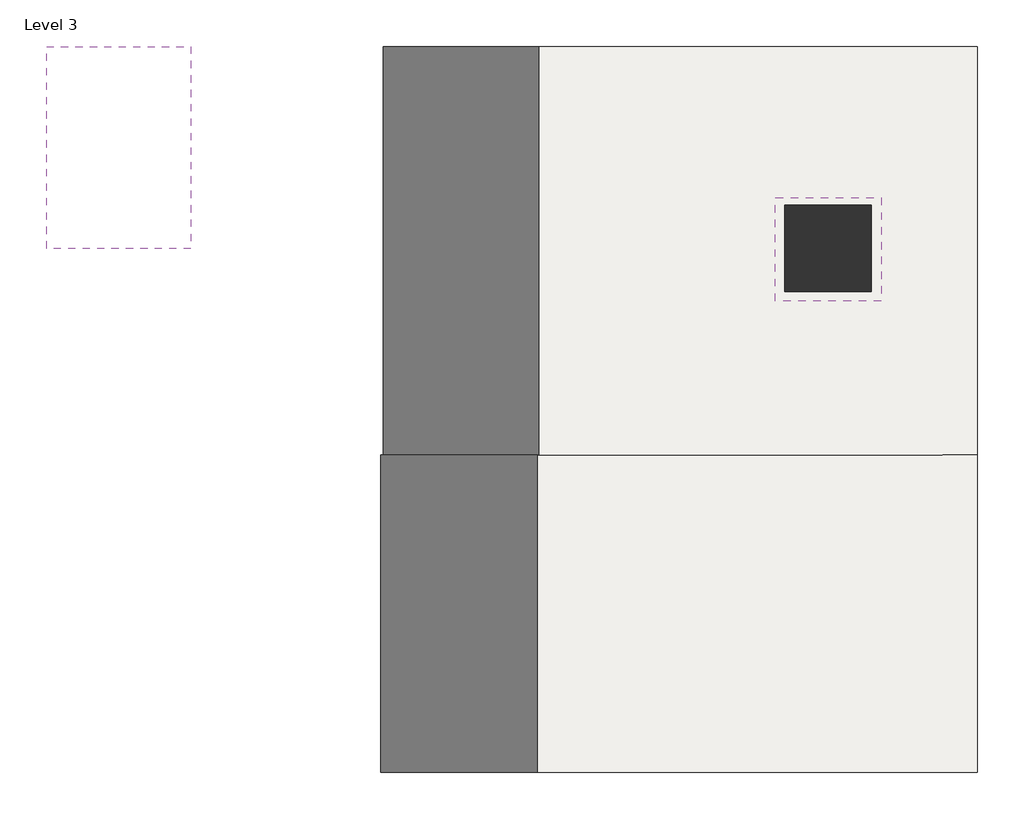
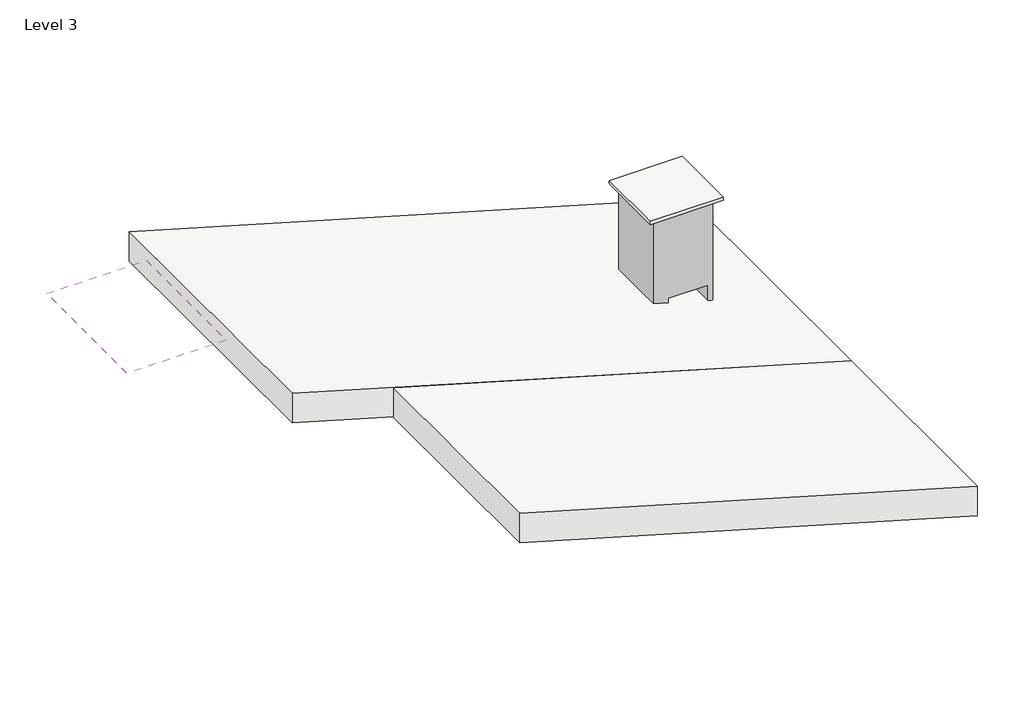
# One storey: 3 roofs, 1 column, 1 slab.
"""IFC4 building model written with IfcOpenShell, lengths in millimetres."""

from ifc_helpers import new_model, si_unit, frame, origin, place, context, project, spatial, polyline, outline, extrude, element, save

model = new_model("IFC4")

# Units and contexts
model_context = context("Model", 3, world=origin())
ifc_project = project(units=[si_unit("LENGTHUNIT", "METRE", prefix="MILLI")], contexts=[model_context])

# Site, building, storey
site = spatial("IfcSite", under=ifc_project)
building = spatial("IfcBuilding", under=site)
storey = spatial("IfcBuildingStorey", under=building, Name="Level 3", Elevation=5181.6)

# Column
placement = place(None, origin())
element("IfcColumn", 1, ObjectType="Rectangular Column : 24\" x 24\" 2", at=placement, inside=storey, context=model_context, shape_type="SweptSolid", body=[
    extrude(outline(polyline([(7010.4, -14282.2613196), (5181.6, -14282.2613196), (5181.6, -14053.6613196), (5638.8, -14053.6613196), (5638.8, -13444.0613196), (5181.6, -13444.0613196), (5181.6, -13367.8613196), (7010.4, -13367.8613196), (7010.4, -14282.2613196)])), frame((0.0, -279.8582127, 0.0), z_axis=(0.0, 1.0, 0.0), x_axis=(0.0, 0.0, 1.0)), (0.0, 0.0, 1.0), 914.4),
])

# Roofs
element("IfcRoof", 2, ObjectType="Generic - 18\"", at=placement, inside=storey, context=model_context, shape_type="SweptSolid", body=[
    extrude(outline(polyline([(5047.6877785, -12248.68247), (7061.3825559, -19259.08247), (6585.6947773, -19259.08247), (4572.0, -12248.68247), (5047.6877785, -12248.68247)])), frame((0.0, -5359.8582127, 0.0), z_axis=(0.0, 1.0, 0.0), x_axis=(0.0, 0.0, 1.0)), (0.0, 0.0, 1.0), 3352.8),
])
element("IfcRoof", 3, ObjectType="Generic - 18\"", at=placement, inside=storey, context=model_context, shape_type="SweptSolid", body=[
    extrude(outline(polyline([(5047.8158981, -12248.68247), (7515.766207, -20810.3057456), (7039.9503089, -20810.3057456), (4572.0, -12248.68247), (5047.8158981, -12248.68247)])), frame((0.0, -2007.0582127, 0.0), z_axis=(0.0, 1.0, 0.0), x_axis=(0.0, 0.0, 1.0)), (0.0, 0.0, 1.0), 4318.0),
])
element("IfcRoof", 4, ObjectType="Generic - 18\"", at=placement, inside=storey, context=model_context, shape_type="SweptSolid", body=[
    extrude(outline(polyline([(7441.3615965, -20556.0613196), (7947.571872, -22080.0613196), (7465.8102755, -22080.0613196), (6959.6, -20556.0613196), (7441.3615965, -20556.0613196)])), frame((0.0, 177.3417873, 0.0), z_axis=(0.0, 1.0, 0.0), x_axis=(0.0, 0.0, 1.0)), (0.0, 0.0, 1.0), 2133.6),
])

# Slab
element("IfcSlab", 5, ObjectType="Generic - 12\" 2", at=placement, inside=storey, context=model_context, shape_type="SweptSolid", body=[
    extrude(outline(polyline([(-13264.463748, 713.3946973), (-13264.463748, -378.8053027), (-14382.063748, -378.8053027), (-14382.063748, 713.3946973), (-13264.463748, 713.3946973)])), frame((0.0, 0.0, 7010.4), z_axis=(0.0, 0.0, 1.0), x_axis=(1.0, 0.0, 0.0)), (0.0, 0.0, 1.0), 50.8),
])

save(model, "model.ifc")

# Revit data of these elements
# Type "Rectangular Column : 24\" x 24\" 2"
#   Assembly Code = "B1010200"
#   Depth = 3' - 0"
#   Offset Base = 0' - 0"
#   Offset Top = 0' - 0"
#   Width = 3' - 0"
#   Material = Iron, Ductile
# Type "Generic - 18\""
#   Assembly Code = "B1020"
#   Layers, outside or top first: 1' - 6" "Stainless Steel" (function 1)
# Type "Generic - 12\" 2"
#   Assembly Code = "B1010"
#   Function = 0
#   Layers, outside or top first: 0' - 2" "Vinyl Composition Tile" (function 1)
# Element 1 (IfcColumn, "Rectangular Column : 24\" x 24\" 2")
#   Phase Created = New Construction
#   Materials on its faces: "Iron, Ductile", "Rigid insulation", "Brick, Soldier Course", "Oak Flooring"
# Element 2 (IfcRoof, "Generic - 18\"")
#   built-in parameter 1001705 = 23.1673 (stored number, unit not read)
#   built-in parameter 1001701 = -2 (stored number, unit not read)
#   built-in parameter 1001710 = 33615
#   Phase Created = New Construction
#   Materials on its faces: "Stainless Steel"
# Element 3 (IfcRoof, "Generic - 18\"")
#   built-in parameter 1001705 = 24.658 (stored number, unit not read)
#   built-in parameter 1001701 = -2 (stored number, unit not read)
#   built-in parameter 1001710 = 33615
#   Phase Created = New Construction
#   Materials on its faces: "Stainless Steel"
# Element 4 (IfcRoof, "Generic - 18\"")
#   built-in parameter 1001705 = 26.0747 (stored number, unit not read)
#   built-in parameter 1001701 = 5.83333 (stored number, unit not read)
#   built-in parameter 1001710 = 33615
#   Phase Created = New Construction
#   Materials on its faces: "Stainless Steel"
# Element 5 (IfcSlab, "Generic - 12\" 2")
#   Height Offset From Level = 6' - 2"
#   Phase Created = New Construction
#   Materials on its faces: "Vinyl Composition Tile"
# Materials
#   "Iron, Ductile": class "Metal", colour RGB 0 0 0, transparency 0, Description = "Ductile cast iron", Cost = 0
#   "Stainless Steel": class "Metal", colour RGB 0 0 0, transparency 0, Description = "Stainless Steel 18/8", Cost = 0
#   "Vinyl Composition Tile": class "Generic", colour RGB 179 160 124, transparency 0, Description = "Vinyl Composition Tile", Cost = 0
#   "Rigid insulation": class "Generic", colour RGB 127 127 127, transparency 0, Description = "Rigid foam insulation board", Cost = 0
#   "Brick, Soldier Course": class "Masonry", colour RGB 170 98 104, transparency 0, Description = "Common brick soldier coursed", Cost = 0
#   "Oak Flooring": class "Wood", colour RGB 216 169 114, transparency 0, Description = "Quercus Rubra", Cost = 0
